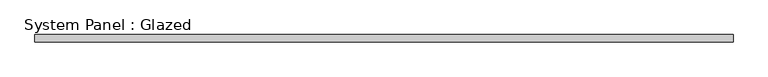
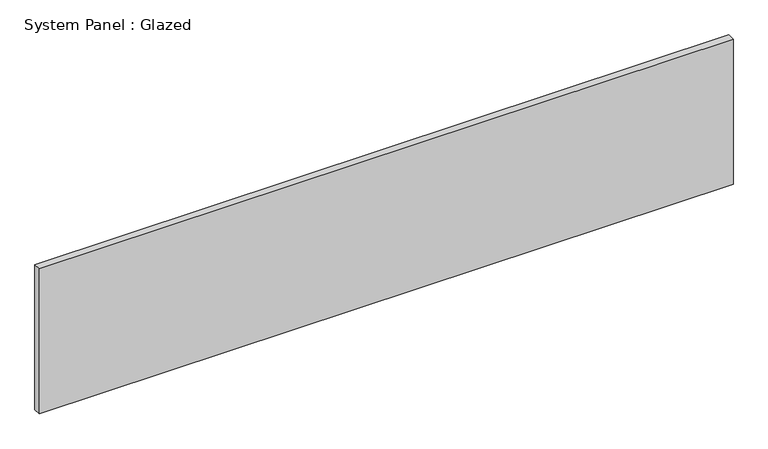
"""IFC4 building model written with IfcOpenShell, lengths in millimetres: plate geometry, System Panel : Glazed."""

from ifc_helpers import new_model, si_unit, origin, origin_with_axes, place, context, project, spatial, polyline, outline, extrude, source, transform, mapped, element, save


def system_panel_glazed_646da070(model_context):
    return source(origin(), model_context, "Body", "SweptSolid", [
        extrude(outline(polyline([(1171.575, 19.05), (-1171.575, 19.05), (-1171.575, 44.45), (1171.575, 44.45), (1171.575, 19.05)])), origin_with_axes(), (0.0, 0.0, 1.0), 517.5437999),
    ])


if __name__ == "__main__":
    model = new_model("IFC4")
    model_context = context("Model", 3, world=origin())
    ifc_project = project(units=[si_unit("LENGTHUNIT", "METRE", prefix="MILLI")], contexts=[model_context])
    site = spatial("IfcSite", under=ifc_project)
    building = spatial("IfcBuilding", under=site)
    placement = place(None, origin())
    system_panel_glazed_shape = system_panel_glazed_646da070(model_context)
    element("IfcPlate", 1, ObjectType="System Panel : Glazed", at=placement, inside=building, context=model_context, shape_type="MappedRepresentation", body=[
        mapped(system_panel_glazed_shape, transform((0.0, 0.0, 0.0), x_axis=(1.0, 0.0, 0.0), y_axis=(0.0, 1.0, 0.0), z_axis=(0.0, 0.0, 1.0))),
    ])
    save(model, "model.ifc")

# Revit data of these elements
# Type "System Panel : Glazed"
#   Construction Type Id = "GSP4R"
#   Analytic Construction = "1/8 in Pilkington single glazing"
#   Visual Light Transmittance = 0.9
#   Solar Heat Gain Coefficient = 0.86
#   Heat Transfer Coefficient (U) = 1.18115 BTU/(h·ft²·°F)
#   Define Thermal Properties by = 1
# Element 1 (IfcPlate, "System Panel : Glazed")
#   Materials on its faces: "Glass"
# Materials
#   "Glass": class "Glass", colour RGB 0 128 192, transparency 0.75, Description = "Soda Lime Glass", Cost = 0
